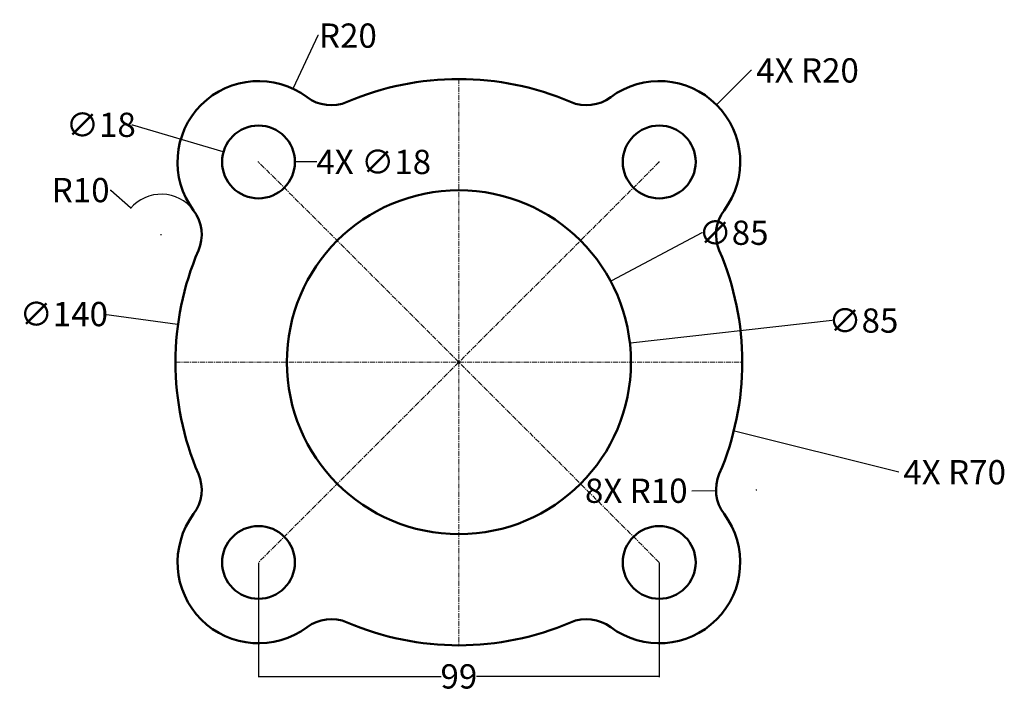
# Model space of a CAD drawing. Units: millimetres. Extents: x 23 to 266, y 65 to 232.
import ezdxf

# ---------------------------------------------------------------- set-up
doc = ezdxf.new("R2010")
doc.units = ezdxf.units.MM
doc.header["$MEASUREMENT"] = 0
doc.linetypes.add('CENTER', pattern=[2, 1.25, -0.25, 0.25, -0.25])
for name, color, linetype, lineweight in [('M-CNTR', 4, 'CENTER', 18), ('M-DIMS', 2, 'Continuous', 25), ('M-OUTL', 7, 'Continuous', 50)]:
    doc.layers.add(name, color=color, linetype=linetype, lineweight=lineweight)
doc.styles.get("Standard").update_dxf_attribs({"font": 'arial.ttf'})
doc.dimstyles.get("Standard").update_dxf_attribs({"dimtxt": 6, "dimasz": 0.18, "dimexe": 0.18, "dimexo": 0.0625, "dimgap": 0.09, "dimtad": 0, "dimtoh": 1, "dimdec": 0, "dimzin": 0, "dimdsep": 46, "dimtxsty": 'Standard', "dimcen": 0.09, "dimadec": 0, "dimazin": 0, "dimtfac": 1, "dimtdec": 0, "dimtofl": 0, "dimtmove": 0, "dimatfit": 3, "dimfxl": 1, "dimtolj": 1, "dimtzin": 0, "dimarcsym": 0})

# ---------------------------------------------------------------- blocks, each defined once
blk = doc.blocks.new('*D1')
at = {"layer": 'Defpoints', "color": 0, "transparency": 16777216}
for p in [(73.49, 199.13), (90.75, 194.03)]:
    blk.add_point(p, dxfattribs=at)
at = {"layer": 'M-DIMS', "color": 0, "lineweight": -2, "transparency": 16777216}
for p, q in [((50.83, 205.76), (51.01, 205.76)), ((51.01, 205.76), (73.31, 199.18)), ((82.03, 196.58), (82.21, 196.58)), ((82.12, 196.49), (82.12, 196.67))]:
    blk.add_line(p, q, dxfattribs=at)
at = {"layer": 'M-DIMS', "color": 0, "transparency": 16777216}
blk.add_solid([(73.32, 199.21), (73.31, 199.15), (73.49, 199.13)], dxfattribs=at)
at = {"layer": 'M-DIMS', "color": 0, "transparency": 16777216, "insert": (43.17, 205.76), "char_height": 6, "attachment_point": 5}
blk.add_mtext('\\A1;∅18', dxfattribs=at)
blk = doc.blocks.new('*D2')
at = {"layer": 'Defpoints', "color": 0, "transparency": 16777216}
for p in [(90.62, 214.68), (82.12, 196.58)]:
    blk.add_point(p, dxfattribs=at)
at = {"layer": 'M-DIMS', "color": 0, "lineweight": -2, "transparency": 16777216}
for p, q in [((96.78, 227.81), (90.69, 214.85)), ((96.96, 227.81), (96.78, 227.81)), ((82.03, 196.58), (82.21, 196.58)), ((82.12, 196.49), (82.12, 196.67))]:
    blk.add_line(p, q, dxfattribs=at)
at = {"layer": 'M-DIMS', "color": 0, "transparency": 16777216}
blk.add_solid([(90.67, 214.86), (90.72, 214.83), (90.62, 214.68)], dxfattribs=at)
at = {"layer": 'M-DIMS', "color": 0, "transparency": 16777216, "insert": (104.21, 227.81), "char_height": 6, "attachment_point": 5}
blk.add_mtext('\\A1;R20', dxfattribs=at)
blk = doc.blocks.new('*D3')
at = {"layer": 'Defpoints', "color": 0, "transparency": 16777216}
for p in [(173.85, 151.79), (89.38, 142.37)]:
    blk.add_point(p, dxfattribs=at)
at = {"layer": 'M-DIMS', "color": 0, "lineweight": -2, "transparency": 16777216}
for p, q in [((223.87, 157.37), (174.03, 151.81)), ((131.53, 147.08), (131.71, 147.08)), ((131.62, 146.99), (131.62, 147.17))]:
    blk.add_line(p, q, dxfattribs=at)
at = {"layer": 'M-DIMS', "color": 0, "transparency": 16777216}
blk.add_solid([(174.03, 151.84), (174.04, 151.78), (173.85, 151.79)], dxfattribs=at)
at = {"layer": 'M-DIMS', "color": 0, "transparency": 16777216, "insert": (231.54, 157.37), "char_height": 6, "attachment_point": 5}
blk.add_mtext('\\A1;∅85', dxfattribs=at)
blk = doc.blocks.new('*D4')
at = {"layer": 'Defpoints', "color": 0, "transparency": 16777216}
for p in [(62.25, 156.5), (200.98, 137.66)]:
    blk.add_point(p, dxfattribs=at)
at = {"layer": 'M-DIMS', "color": 0, "lineweight": -2, "transparency": 16777216}
for p, q in [((44.01, 158.98), (62.07, 156.52)), ((131.53, 147.08), (131.71, 147.08)), ((131.62, 146.99), (131.62, 147.17))]:
    blk.add_line(p, q, dxfattribs=at)
at = {"layer": 'M-DIMS', "color": 0, "transparency": 16777216}
blk.add_solid([(62.08, 156.55), (62.07, 156.5), (62.25, 156.5)], dxfattribs=at)
at = {"layer": 'M-DIMS', "color": 0, "transparency": 16777216, "insert": (34.03, 158.98), "char_height": 6, "attachment_point": 5}
blk.add_mtext('\\A1;∅140', dxfattribs=at)
blk = doc.blocks.new('*D5')
at = {"layer": 'Defpoints', "color": 0, "transparency": 16777216}
for p in [(50.6, 185.23), (58.09, 178.61)]:
    blk.add_point(p, dxfattribs=at)
at = {"layer": 'M-DIMS', "color": 0, "lineweight": -2, "transparency": 16777216}
for p, q in [((45.44, 189.63), (45.62, 189.63)), ((45.62, 189.63), (50.46, 185.35)), ((58, 178.61), (58.18, 178.61)), ((58.09, 178.52), (58.09, 178.7))]:
    blk.add_line(p, q, dxfattribs=at)
blk.add_arc((58.09, 178.61), 10, 37.1449, 139.5692, dxfattribs=at)
at = {"layer": 'M-DIMS', "color": 0, "transparency": 16777216}
blk.add_solid([(50.48, 185.38), (50.44, 185.33), (50.6, 185.23)], dxfattribs=at)
at = {"layer": 'M-DIMS', "color": 0, "transparency": 16777216, "insert": (38.19, 189.63), "char_height": 6, "attachment_point": 5}
blk.add_mtext('\\A1;R10', dxfattribs=at)
blk = doc.blocks.new('MOUNT-HOLE-D18')
blk.add_circle((9, 9), 9)
blk = doc.blocks.new('*D7')
at = {"layer": 'Defpoints', "color": 0, "transparency": 16777216}
for p in [(82.12, 97.58), (181.11, 97.58), (181.11, 69.41)]:
    blk.add_point(p, dxfattribs=at)
at = {"layer": 'M-DIMS', "color": 0, "lineweight": -2, "transparency": 16777216}
for p, q in [((82.12, 97.52), (82.12, 69.23)), ((181.11, 97.52), (181.11, 69.23)), ((82.3, 69.41), (127.22, 69.41)), ((180.93, 69.41), (136.01, 69.41))]:
    blk.add_line(p, q, dxfattribs=at)
at = {"layer": 'M-DIMS', "color": 0, "transparency": 16777216}
for points in [[(82.3, 69.44), (82.3, 69.38), (82.12, 69.41)], [(180.93, 69.44), (180.93, 69.38), (181.11, 69.41)]]:
    blk.add_solid(points, dxfattribs=at)
at = {"layer": 'M-DIMS', "color": 0, "transparency": 16777216, "insert": (131.62, 69.41), "char_height": 6, "attachment_point": 5}
blk.add_mtext('\\A1;99', dxfattribs=at)
blk = doc.blocks.new('*D8')
at = {"layer": 'Defpoints', "color": 0, "transparency": 16777216}
for p in [(131.62, 147.08), (199.52, 130.08)]:
    blk.add_point(p, dxfattribs=at)
at = {"layer": 'M-DIMS', "color": 0, "lineweight": -2, "transparency": 16777216}
for p, q in [((131.53, 147.08), (131.71, 147.08)), ((131.62, 146.99), (131.62, 147.17)), ((240.26, 119.88), (199.69, 130.04))]:
    blk.add_line(p, q, dxfattribs=at)
at = {"layer": 'M-DIMS', "color": 0, "transparency": 16777216}
blk.add_solid([(199.7, 130.07), (199.69, 130.01), (199.52, 130.08)], dxfattribs=at)
at = {"layer": 'M-DIMS', "color": 0, "transparency": 16777216, "insert": (254.08, 119.88), "char_height": 6, "attachment_point": 5}
blk.add_mtext('\\A1;4X R70', dxfattribs=at)
blk = doc.blocks.new('*D9')
at = {"layer": 'Defpoints', "color": 0, "transparency": 16777216}
for p in [(169.12, 167.08), (94.11, 127.08)]:
    blk.add_point(p, dxfattribs=at)
at = {"layer": 'M-DIMS', "color": 0, "lineweight": -2, "transparency": 16777216}
for p, q in [((191.62, 179.08), (169.28, 167.16)), ((191.8, 179.08), (191.62, 179.08)), ((131.53, 147.08), (131.71, 147.08)), ((131.62, 146.99), (131.62, 147.17))]:
    blk.add_line(p, q, dxfattribs=at)
at = {"layer": 'M-DIMS', "color": 0, "transparency": 16777216}
blk.add_solid([(169.26, 167.19), (169.29, 167.14), (169.12, 167.08)], dxfattribs=at)
at = {"layer": 'M-DIMS', "color": 0, "transparency": 16777216, "insert": (199.47, 179.08), "char_height": 6, "attachment_point": 5}
blk.add_mtext('\\A1;∅85', dxfattribs=at)
blk = doc.blocks.new('*D10')
at = {"layer": 'Defpoints', "color": 0, "transparency": 16777216}
for p in [(73.12, 196.58), (91.12, 196.58)]:
    blk.add_point(p, dxfattribs=at)
at = {"layer": 'M-DIMS', "color": 0, "lineweight": -2, "transparency": 16777216}
for p, q in [((82.03, 196.58), (82.21, 196.58)), ((82.12, 196.49), (82.12, 196.67)), ((96.52, 196.58), (91.3, 196.58))]:
    blk.add_line(p, q, dxfattribs=at)
at = {"layer": 'M-DIMS', "color": 0, "transparency": 16777216}
blk.add_solid([(91.3, 196.61), (91.3, 196.55), (91.12, 196.58)], dxfattribs=at)
at = {"layer": 'M-DIMS', "color": 0, "transparency": 16777216, "insert": (110.58, 196.58), "char_height": 6, "attachment_point": 5}
blk.add_mtext('\\A1;4X ∅18', dxfattribs=at)
blk = doc.blocks.new('*D11')
at = {"layer": 'Defpoints', "color": 0, "transparency": 16777216}
for p in [(195.26, 210.72), (181.11, 196.58)]:
    blk.add_point(p, dxfattribs=at)
at = {"layer": 'M-DIMS', "color": 0, "lineweight": -2, "transparency": 16777216}
for p, q in [((203.74, 219.21), (195.38, 210.85)), ((203.92, 219.21), (203.74, 219.21)), ((181.02, 196.58), (181.2, 196.58)), ((181.11, 196.49), (181.11, 196.67))]:
    blk.add_line(p, q, dxfattribs=at)
at = {"layer": 'M-DIMS', "color": 0, "transparency": 16777216}
blk.add_solid([(195.36, 210.87), (195.4, 210.83), (195.26, 210.72)], dxfattribs=at)
at = {"layer": 'M-DIMS', "color": 0, "transparency": 16777216, "insert": (217.74, 219.21), "char_height": 6, "attachment_point": 5}
blk.add_mtext('\\A1;4X R20', dxfattribs=at)
blk = doc.blocks.new('*D12')
at = {"layer": 'Defpoints', "color": 0, "transparency": 16777216}
for p in [(195.14, 115.4), (205.14, 115.55)]:
    blk.add_point(p, dxfattribs=at)
at = {"layer": 'M-DIMS', "color": 0, "lineweight": -2, "transparency": 16777216}
for p, q in [((189.14, 115.31), (194.96, 115.4)), ((205.05, 115.55), (205.23, 115.55)), ((205.14, 115.46), (205.14, 115.64))]:
    blk.add_line(p, q, dxfattribs=at)
at = {"layer": 'M-DIMS', "color": 0, "transparency": 16777216}
blk.add_solid([(194.96, 115.43), (194.96, 115.37), (195.14, 115.4)], dxfattribs=at)
at = {"layer": 'M-DIMS', "color": 0, "transparency": 16777216, "insert": (175.44, 115.31), "char_height": 6, "attachment_point": 5}
blk.add_mtext('\\A1;8X R10', dxfattribs=at)

msp = doc.modelspace()

# ---------------------------------------------------------------- linework, layer by layer
at = {"layer": 'M-CNTR'}
for p, q in [((131.62, 217.08), (131.62, 77.08)), ((181.11, 97.58), (82.12, 196.58)), ((181.11, 196.58), (82.12, 97.58)), ((61.62, 147.08), (201.62, 147.08))]:
    msp.add_line(p, q, dxfattribs=at)
at = {"layer": 'M-OUTL'}
msp.add_lwpolyline([(195.95, 119.49, 0.267949), (197.13, 109.56, -0.866025), (169.14, 81.57, 0.267949), (159.21, 82.75, -0.205391), (104.03, 82.75, 0.267949), (94.1, 81.57, -0.866025), (66.1, 109.56, 0.267949), (67.28, 119.49, -0.205391), (67.28, 174.67, 0.267949), (66.1, 184.6, -0.866025), (94.1, 212.6, 0.267949), (104.03, 211.41, -0.205391), (159.21, 211.41, 0.267949), (169.14, 212.6, -0.866025), (197.13, 184.6, 0.267949), (195.95, 174.67, -0.205391)], format="xyb", close=True, dxfattribs=at)
msp.add_circle((131.62, 147.08), 42.5, dxfattribs=at)

# ---------------------------------------------------------------- block references
for p in [(73.12, 187.58), (172.11, 187.58), (73.12, 88.58), (172.11, 88.58)]:
    msp.add_blockref('MOUNT-HOLE-D18', p, dxfattribs=at)

# ---------------------------------------------------------------- dimensions: what is measured, and where the dimension line sits
at = {"layer": 'M-DIMS'}
for center, mpoint, picture, middle in [((82.12, 196.58), (90.62, 214.68), '*D2', (104.21, 227.81)), ((58.09, 178.61), (50.6, 185.23), '*D5', (38.19, 189.63))]:
    dim = msp.add_radius_dim(center=center, mpoint=mpoint, dimstyle='Standard', override={"dimclrd": 0, "dimclre": 0, "dimclrt": 0}, dxfattribs=at)
    dim.commit()
    dim.dimension.update_dxf_attribs({"geometry": picture, "text_midpoint": middle, "dimtype": 164})
for center, mpoint, text, picture, middle in [((181.11, 196.58), (195.26, 210.72), '4X <>', '*D11', (217.74, 219.21)), ((131.62, 147.08), (199.52, 130.08), '4X <>', '*D8', (240.26, 119.88)), ((205.14, 115.55), (195.14, 115.4), '8X <>', '*D12', (189.14, 115.31))]:
    dim = msp.add_radius_dim(center=center, mpoint=mpoint, text=text, dimstyle='Standard', override={"dimdec": 0, "dimlfac": 1, "dimrnd": 0, "dimzin": 0, "dimdsep": 46, "dimlunit": 2}, dxfattribs=at)
    dim.commit()
    dim.dimension.update_dxf_attribs({"geometry": picture, "text_midpoint": middle, "dimtype": 164})
for p1, p2, override, picture, middle in [((90.75, 194.03), (73.49, 199.13), {"dimclrd": 0, "dimclre": 0, "dimclrt": 0}, '*D1', (43.17, 205.76)), ((94.11, 127.08), (169.12, 167.08), {"dimdec": 0, "dimlfac": 1, "dimrnd": 0, "dimzin": 0, "dimdsep": 46, "dimlunit": 2}, '*D9', (199.47, 179.08)), ((200.98, 137.66), (62.25, 156.5), {"dimclrd": 0, "dimclre": 0, "dimclrt": 0}, '*D4', (44.01, 158.98)), ((89.38, 142.37), (173.85, 151.79), {"dimclrd": 0, "dimclre": 0, "dimclrt": 0}, '*D3', (223.87, 157.37))]:
    dim = msp.add_diameter_dim_2p(p1=p1, p2=p2, dimstyle='Standard', override=override, dxfattribs=at)
    dim.commit()
    dim.dimension.update_dxf_attribs({"geometry": picture, "text_midpoint": middle, "dimtype": 163})
dim = msp.add_diameter_dim_2p(p1=(73.12, 196.58), p2=(91.12, 196.58), text='4X <>', dimstyle='Standard', override={"dimdec": 0, "dimlfac": 1, "dimrnd": 0, "dimzin": 0, "dimdsep": 46, "dimlunit": 2}, dxfattribs=at)
dim.commit()
dim.dimension.update_dxf_attribs({"geometry": '*D10', "text_midpoint": (96.52, 196.58), "dimtype": 163})
dim = msp.add_linear_dim(base=(181.11, 69.41), p1=(82.12, 97.58), p2=(181.11, 97.58), dimstyle='Standard', override={"dimdec": 0, "dimlfac": 1, "dimrnd": 0, "dimzin": 0, "dimdsep": 46, "dimlunit": 2}, dxfattribs=at)
dim.commit()
dim.dimension.update_dxf_attribs({"geometry": '*D7', "text_midpoint": (131.62, 69.41)})

doc.saveas('drawing.dxf')
